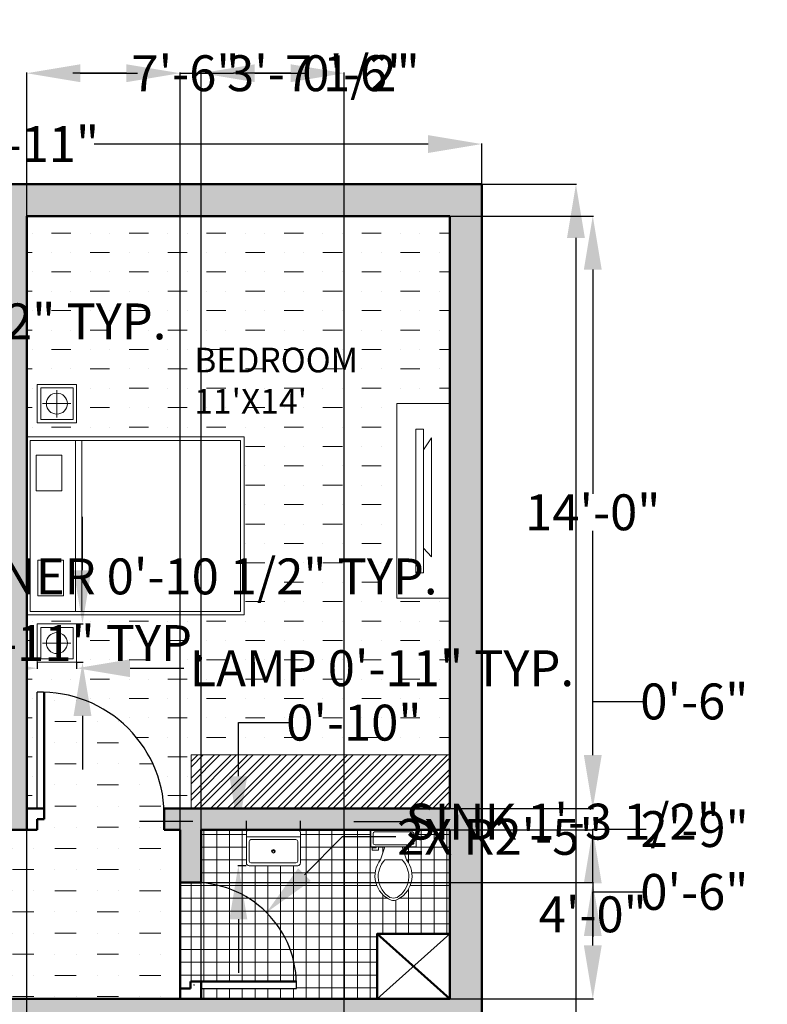
# Model space of a CAD drawing. Units: inches. Extents: x 26 to 14419, y 2 to 3479.
# Tile 5 of 9: x 13791 to 14003, y 3199 to 3479. Entities that reach past the tile are written whole.
import ezdxf

# ---------------------------------------------------------------- set-up
doc = ezdxf.new("R2010")
doc.units = ezdxf.units.IN
doc.header["$MEASUREMENT"] = 0
for name, color, linetype, lineweight in [('A-ANNO-DIMS', 2, 'Continuous', 18), ('A-AREA-IDEN', 7, 'Continuous', 18), ('A-DOOR', 4, 'Continuous', 25), ('A-FLOR-FIXT', 8, 'Continuous', 18), ('A-FLOR-PATT', 252, 'Continuous', 13), ('A-FURN', 8, 'Continuous', 18), ('A-WALL', 7, 'Continuous', 50)]:
    doc.layers.add(name, color=color, linetype=linetype, lineweight=lineweight)
doc.styles.get("Standard").update_dxf_attribs({"font": 'arial.ttf'})
doc.dimstyles.get("Standard").update_dxf_attribs({"dimtxt": 10.18, "dimasz": 15.18, "dimexe": 0.18, "dimexo": 0.0625, "dimgap": 0.09, "dimtad": 0, "dimtih": 1, "dimtoh": 1, "dimdec": 0, "dimzin": 0, "dimdsep": 46, "dimlunit": 3, "dimtxsty": 'Standard', "dimcen": 0.09, "dimadec": 0, "dimazin": 0, "dimtfac": 1, "dimtdec": 0, "dimtofl": 0, "dimtmove": 0, "dimatfit": 3, "dimfxl": 1, "dimtolj": 1, "dimtzin": 0, "dimarcsym": 0})
pattern_1 = [(0, (61.0932, 57.669), (0, 3.625), []), (90, (61.0932, 57.669), (-3.625, 2e-16), [])]

# ---------------------------------------------------------------- blocks, each defined once
blk = doc.blocks.new('*U2')
for p, q in [((9.5, -6), (9.5, -2)), ((-10, -8.5), (-8, -8.5)), ((-10, -9.5), (-10, -8.5)), ((-8, -8.5), (-8, -8)), ((-7, -8), (-7, -9.5)), ((-4, -8), (-6, -14)), ((4, -8), (6, -14)), ((-7, -9.5), (-10, -9.5)), ((4, -14), (-4, -14))]:
    blk.add_line(p, q)
blk.add_lwpolyline([(10.5, -8), (10.5, 0), (-10.5, 0), (-10.5, -8)], close=True)
for points in [[(-9.5, -2), (-9.5, -6)], [(8.5, -1), (-8.5, -1)], [(-8.5, -7), (8.5, -7)]]:
    blk.add_lwpolyline(points)
for centre, radius, start, end in [((-8.62, -1.88), 0.884, 81.8699, 188.1301), ((8.62, -1.88), 0.884, 351.8699, 98.1301), ((-8.62, -6.12), 0.884, 171.8699, 278.1301), ((8.62, -6.12), 0.884, 261.8699, 8.1301), ((3.52, -21.58), 12.17, 141.4691, 247.9714), ((4.2, -21.82), 11.33, 136.3677, 238.9468), ((-3.52, -21.58), 12.17, 292.0284, 38.5307), ((-4.2, -21.82), 11.33, 301.053, 43.6321), ((0, -27.88), 4, 245.7318, 294.2682), ((0, -29), 4, 254.8605, 285.1395)]:
    blk.add_arc(centre, radius, start, end)
blk = doc.blocks.new('Sink-single - 30 in top')
blk.add_line((-15, -3.999996), (15, -3.999996))
for points in [[(-13.5, 0), (13.5, 0)], [(-15, -18.499996), (-15, -1.5)], [(15, -1.5), (15, -18.499996)], [(-13.5, -17.499996), (-13.5, -6.499996)], [(-12.5, -5.499996), (12.5, -5.499996)], [(13.5, -6.499996), (13.5, -17.499996)], [(13.5, -19.999996), (-13.5, -19.999996)], [(12.5, -18.499996), (-12.5, -18.499996)]]:
    blk.add_lwpolyline(points)
for radius in [1, 0.5]:
    blk.add_circle((0, -11.999996), radius)
for centre, radius, start, end in [((-13.5, -1.5), 1.5, 90, 180), ((13.5, -1.5), 1.5, 0, 90), ((-12.5, -6.499996), 1, 90, 180), ((12.5, -6.499996), 1, 0, 90), ((-13.5, -18.499996), 1.5, 180, 270), ((-12.5, -17.499996), 1, 180, 270), ((12.5, -17.499996), 1, 270, 0), ((13.5, -18.499996), 1.5, 270, 0)]:
    blk.add_arc(centre, radius, start, end)
blk = doc.blocks.new('*D6')
at = {"layer": 'A-ANNO-DIMS', "color": 0, "lineweight": -2, "transparency": 16777216}
for p, q in [((13659.09, 3432.06), (13659.09, 3443.59)), ((13674.27, 3443.41), (13768.97, 3443.41)), ((13906.91, 3443.41), (13812.21, 3443.41)), ((13922.09, 3432.06), (13922.09, 3443.59))]:
    blk.add_line(p, q, dxfattribs=at)
at = {"layer": 'A-ANNO-DIMS', "color": 0, "transparency": 16777216}
for points in [[(13674.27, 3445.94), (13674.27, 3440.88), (13659.09, 3443.41)], [(13906.91, 3445.94), (13906.91, 3440.88), (13922.09, 3443.41)]]:
    blk.add_solid(points, dxfattribs=at)
at = {"layer": 'Defpoints', "color": 0, "transparency": 16777216}
for p in [(13922.09, 3443.41), (13659.09, 3432), (13922.09, 3432)]:
    blk.add_point(p, dxfattribs=at)
at = {"layer": 'A-ANNO-DIMS', "color": 0, "transparency": 16777216, "insert": (13790.59, 3443.41), "char_height": 10.18, "attachment_point": 5}
blk.add_mtext('\\A1;21\'-11"', dxfattribs=at)
blk = doc.blocks.new('*D7')
at = {"layer": 'A-ANNO-DIMS', "color": 0, "lineweight": -2, "transparency": 16777216}
for p, q in [((13922.15, 3432), (13949, 3432)), ((13948.82, 3416.82), (13948.82, 3142.28)), ((13948.82, 2857.18), (13948.82, 3131.71)), ((13922.15, 2842), (13949, 2842))]:
    blk.add_line(p, q, dxfattribs=at)
at = {"layer": 'A-ANNO-DIMS', "color": 0, "transparency": 16777216}
for points in [[(13946.29, 3416.82), (13951.35, 3416.82), (13948.82, 3432)], [(13946.29, 2857.18), (13951.35, 2857.18), (13948.82, 2842)]]:
    blk.add_solid(points, dxfattribs=at)
at = {"layer": 'Defpoints', "color": 0, "transparency": 16777216}
for p in [(13922.09, 3432), (13922.09, 2842), (13948.82, 2842)]:
    blk.add_point(p, dxfattribs=at)
at = {"layer": 'A-ANNO-DIMS', "color": 0, "transparency": 16777216, "insert": (13948.82, 3137), "char_height": 10.18, "attachment_point": 5}
blk.add_mtext('\\A1;49\'-2"', dxfattribs=at)
blk = doc.blocks.new('DOOR-900')
blk.add_line((0, 3), (0, 36))
blk.add_arc((1, 1), 35.01, 358.3634, 91.6366)
blk = doc.blocks.new('DOOR-750')
blk.add_line((3, 0), (30, 0))
blk.add_arc((1, 1), 29.02, 358.0251, 91.9749)
blk = doc.blocks.new('LAMP')
for p, q in [((5.59, 9.24), (5.59, 1.57)), ((1.47, 5.46), (9.59, 5.46))]:
    blk.add_line(p, q)
for points in [[(0, 10.91), (11.18, 10.91), (11.18, 0), (0, 0)], [(1, 9.91), (10.18, 9.91), (10.18, 1), (1, 1)]]:
    blk.add_lwpolyline(points, close=True)
blk.add_circle((5.59, 5.46), 2.98)
blk = doc.blocks.new('*D24')
at = {"layer": 'A-ANNO-DIMS', "color": 0, "lineweight": -2, "transparency": 16777216}
for p, q in [((13730.53, 3172.73), (13730.53, 3187.91)), ((13730.53, 3187.91), (13745.71, 3187.91)), ((13728.71, 3157.55), (13730.71, 3157.55)), ((13728.71, 3147.87), (13730.71, 3147.87)), ((13730.53, 3132.69), (13730.53, 3117.51))]:
    blk.add_line(p, q, dxfattribs=at)
at = {"layer": 'A-ANNO-DIMS', "color": 0, "transparency": 16777216}
for points in [[(13728, 3172.73), (13733.06, 3172.73), (13730.53, 3157.55)], [(13728, 3132.69), (13733.06, 3132.69), (13730.53, 3147.87)]]:
    blk.add_solid(points, dxfattribs=at)
at = {"layer": 'Defpoints', "color": 0, "transparency": 16777216}
for p in [(13728.65, 3157.55), (13730.53, 3157.55), (13728.65, 3147.87)]:
    blk.add_point(p, dxfattribs=at)
at = {"layer": 'A-ANNO-DIMS', "color": 0, "transparency": 16777216, "insert": (13788.69, 3187.91), "char_height": 10.18, "attachment_point": 5}
blk.add_mtext('\\A1;0\'-9 1/2" TYP.', dxfattribs=at)
blk = doc.blocks.new('*D27')
at = {"layer": 'A-ANNO-DIMS', "color": 0, "lineweight": -2, "transparency": 16777216}
for p, q in [((13755.48, 3423.45), (13755.48, 3438.63)), ((13751.01, 3408.27), (13755.66, 3408.27)), ((13751.01, 3378), (13755.66, 3378)), ((13755.48, 3362.82), (13755.48, 3347.64))]:
    blk.add_line(p, q, dxfattribs=at)
at = {"layer": 'A-ANNO-DIMS', "color": 0, "transparency": 16777216}
for points in [[(13752.95, 3423.45), (13758.01, 3423.45), (13755.48, 3408.27)], [(13752.95, 3362.82), (13758.01, 3362.82), (13755.48, 3378)]]:
    blk.add_solid(points, dxfattribs=at)
at = {"layer": 'Defpoints', "color": 0, "transparency": 16777216}
for p in [(13750.94, 3408.27), (13755.48, 3408.27), (13750.94, 3378)]:
    blk.add_point(p, dxfattribs=at)
at = {"layer": 'A-ANNO-DIMS', "color": 0, "transparency": 16777216, "insert": (13755.48, 3393.13), "char_height": 10.18, "attachment_point": 5}
blk.add_mtext('\\A1;DOOR 750 2\'-6 1/2" TYP.', dxfattribs=at)
blk = doc.blocks.new('*D35')
at = {"layer": 'A-ANNO-DIMS', "color": 0, "lineweight": -2, "transparency": 16777216}
for p, q in [((13780.88, 3294.79), (13765.7, 3294.79)), ((13796.06, 3296.4), (13796.06, 3294.61)), ((13807.24, 3296.4), (13807.24, 3294.61)), ((13822.42, 3294.79), (13837.6, 3294.79))]:
    blk.add_line(p, q, dxfattribs=at)
at = {"layer": 'A-ANNO-DIMS', "color": 0, "transparency": 16777216}
for points in [[(13780.88, 3297.32), (13780.88, 3292.26), (13796.06, 3294.79)], [(13822.42, 3297.32), (13822.42, 3292.26), (13807.24, 3294.79)]]:
    blk.add_solid(points, dxfattribs=at)
at = {"layer": 'Defpoints', "color": 0, "transparency": 16777216}
for p in [(13796.06, 3296.46), (13807.24, 3296.46), (13807.24, 3294.79)]:
    blk.add_point(p, dxfattribs=at)
at = {"layer": 'A-ANNO-DIMS', "color": 0, "transparency": 16777216, "insert": (13893.78, 3294.79), "char_height": 10.18, "attachment_point": 5}
blk.add_mtext('\\A1;LAMP 0\'-11" TYP.', dxfattribs=at)
blk = doc.blocks.new('*D36')
at = {"layer": 'A-ANNO-DIMS', "color": 0, "lineweight": -2, "transparency": 16777216}
for p, q in [((13808.91, 3322.56), (13808.91, 3337.74)), ((13807.3, 3307.38), (13809.09, 3307.38)), ((13807.3, 3296.46), (13809.09, 3296.46)), ((13808.91, 3281.28), (13808.91, 3266.1))]:
    blk.add_line(p, q, dxfattribs=at)
at = {"layer": 'A-ANNO-DIMS', "color": 0, "transparency": 16777216}
for points in [[(13806.38, 3322.56), (13811.44, 3322.56), (13808.91, 3307.38)], [(13806.38, 3281.28), (13811.44, 3281.28), (13808.91, 3296.46)]]:
    blk.add_solid(points, dxfattribs=at)
at = {"layer": 'Defpoints', "color": 0, "transparency": 16777216}
for p in [(13807.24, 3307.38), (13808.91, 3307.38), (13807.24, 3296.46)]:
    blk.add_point(p, dxfattribs=at)
at = {"layer": 'A-ANNO-DIMS', "color": 0, "transparency": 16777216, "insert": (13808.91, 3301.92), "char_height": 10.18, "attachment_point": 5}
blk.add_mtext('\\A1;0\'-11" TYP.', dxfattribs=at)
blk = doc.blocks.new('*D47')
at = {"layer": 'A-ANNO-DIMS', "color": 0, "lineweight": -2, "transparency": 16777216}
for p, q in [((13680.17, 3322.36), (13680.17, 3320.64)), ((13690.89, 3322.36), (13690.89, 3320.64)), ((13664.99, 3320.82), (13649.81, 3320.82)), ((13706.07, 3320.82), (13721.25, 3320.82))]:
    blk.add_line(p, q, dxfattribs=at)
at = {"layer": 'A-ANNO-DIMS', "color": 0, "transparency": 16777216}
for points in [[(13664.99, 3323.35), (13664.99, 3318.29), (13680.17, 3320.82)], [(13706.07, 3323.35), (13706.07, 3318.29), (13690.89, 3320.82)]]:
    blk.add_solid(points, dxfattribs=at)
at = {"layer": 'Defpoints', "color": 0, "transparency": 16777216}
for p in [(13680.17, 3322.43), (13690.89, 3322.43), (13690.89, 3320.82)]:
    blk.add_point(p, dxfattribs=at)
at = {"layer": 'A-ANNO-DIMS', "color": 0, "transparency": 16777216, "insert": (13817.29, 3320.82), "char_height": 10.18, "attachment_point": 5}
blk.add_mtext('\\A1;HOB BURNER 0\'-10 1/2" TYP.', dxfattribs=at)
blk = doc.blocks.new('*D49')
at = {"layer": 'A-ANNO-DIMS', "color": 0, "lineweight": -2, "transparency": 16777216}
for p, q in [((13840.22, 3251.29), (13825.04, 3251.29)), ((13855.4, 3249.06), (13855.4, 3251.47)), ((13870.71, 3249.06), (13870.71, 3251.47)), ((13885.89, 3251.29), (13901.07, 3251.29))]:
    blk.add_line(p, q, dxfattribs=at)
at = {"layer": 'A-ANNO-DIMS', "color": 0, "transparency": 16777216}
for points in [[(13840.22, 3253.82), (13840.22, 3248.76), (13855.4, 3251.29)], [(13885.89, 3253.82), (13885.89, 3248.76), (13870.71, 3251.29)]]:
    blk.add_solid(points, dxfattribs=at)
at = {"layer": 'Defpoints', "color": 0, "transparency": 16777216}
for p in [(13870.71, 3251.29), (13855.4, 3249), (13870.71, 3249)]:
    blk.add_point(p, dxfattribs=at)
at = {"layer": 'A-ANNO-DIMS', "color": 0, "transparency": 16777216, "insert": (13945.09, 3251.29), "char_height": 10.18, "attachment_point": 5}
blk.add_mtext('\\A1;SINK 1\'-3 1/2"', dxfattribs=at)
blk = doc.blocks.new('*D50')
at = {"layer": 'A-ANNO-DIMS', "color": 0, "lineweight": -2, "transparency": 16777216}
for p, q in [((13853.1, 3264.18), (13853.1, 3279.36)), ((13853.1, 3279.36), (13868.28, 3279.36)), ((13855.34, 3249), (13852.92, 3249)), ((13855.34, 3238.79), (13852.92, 3238.79)), ((13853.1, 3223.61), (13853.1, 3208.43))]:
    blk.add_line(p, q, dxfattribs=at)
at = {"layer": 'A-ANNO-DIMS', "color": 0, "transparency": 16777216}
for points in [[(13850.57, 3264.18), (13855.63, 3264.18), (13853.1, 3249)], [(13850.57, 3223.61), (13855.63, 3223.61), (13853.1, 3238.79)]]:
    blk.add_solid(points, dxfattribs=at)
at = {"layer": 'Defpoints', "color": 0, "transparency": 16777216}
for p in [(13853.1, 3249), (13855.4, 3249), (13855.4, 3238.79)]:
    blk.add_point(p, dxfattribs=at)
at = {"layer": 'A-ANNO-DIMS', "color": 0, "transparency": 16777216, "insert": (13885.86, 3279.36), "char_height": 10.18, "attachment_point": 5}
blk.add_mtext('\\A1;0\'-10"', dxfattribs=at)
blk = doc.blocks.new('*D68')
at = {"layer": 'A-ANNO-DIMS', "color": 0, "lineweight": -2, "transparency": 16777216}
for p, q in [((13953.59, 3216.18), (13953.59, 3231.36)), ((13953.59, 3231.36), (13968.77, 3231.36)), ((13913.15, 3201), (13953.77, 3201)), ((13913.15, 3195), (13953.77, 3195)), ((13953.59, 3179.82), (13953.59, 3164.64))]:
    blk.add_line(p, q, dxfattribs=at)
at = {"layer": 'A-ANNO-DIMS', "color": 0, "transparency": 16777216}
for points in [[(13951.06, 3216.18), (13956.12, 3216.18), (13953.59, 3201)], [(13951.06, 3179.82), (13956.12, 3179.82), (13953.59, 3195)]]:
    blk.add_solid(points, dxfattribs=at)
at = {"layer": 'Defpoints', "color": 0, "transparency": 16777216}
for p in [(13913.09, 3201), (13953.59, 3201), (13913.09, 3195)]:
    blk.add_point(p, dxfattribs=at)
at = {"layer": 'A-ANNO-DIMS', "color": 0, "transparency": 16777216, "insert": (13982.39, 3231.36), "char_height": 10.18, "attachment_point": 5}
blk.add_mtext('\\A1;0\'-6"', dxfattribs=at)
blk = doc.blocks.new('*D69')
at = {"layer": 'A-ANNO-DIMS', "color": 0, "lineweight": -2, "transparency": 16777216}
for p, q in [((13913.15, 3249), (13953.77, 3249)), ((13953.59, 3233.82), (13953.59, 3230.28)), ((13953.59, 3216.18), (13953.59, 3219.71)), ((13913.15, 3201), (13953.77, 3201))]:
    blk.add_line(p, q, dxfattribs=at)
at = {"layer": 'A-ANNO-DIMS', "color": 0, "transparency": 16777216}
for points in [[(13951.06, 3233.82), (13956.12, 3233.82), (13953.59, 3249)], [(13951.06, 3216.18), (13956.12, 3216.18), (13953.59, 3201)]]:
    blk.add_solid(points, dxfattribs=at)
at = {"layer": 'Defpoints', "color": 0, "transparency": 16777216}
for p in [(13913.09, 3249), (13953.59, 3249), (13913.09, 3201)]:
    blk.add_point(p, dxfattribs=at)
at = {"layer": 'A-ANNO-DIMS', "color": 0, "transparency": 16777216, "insert": (13953.59, 3225), "char_height": 10.18, "attachment_point": 5}
blk.add_mtext('\\A1;4\'-0"', dxfattribs=at)
blk = doc.blocks.new('*D70')
at = {"layer": 'A-ANNO-DIMS', "color": 0, "lineweight": -2, "transparency": 16777216}
for p, q in [((13953.59, 3270.18), (13953.59, 3285.36)), ((13953.59, 3285.36), (13968.77, 3285.36)), ((13913.15, 3255), (13953.77, 3255)), ((13913.15, 3249), (13953.77, 3249)), ((13953.59, 3233.82), (13953.59, 3218.64))]:
    blk.add_line(p, q, dxfattribs=at)
at = {"layer": 'A-ANNO-DIMS', "color": 0, "transparency": 16777216}
for points in [[(13951.06, 3270.18), (13956.12, 3270.18), (13953.59, 3255)], [(13951.06, 3233.82), (13956.12, 3233.82), (13953.59, 3249)]]:
    blk.add_solid(points, dxfattribs=at)
at = {"layer": 'Defpoints', "color": 0, "transparency": 16777216}
for p in [(13913.09, 3255), (13953.59, 3255), (13913.09, 3249)]:
    blk.add_point(p, dxfattribs=at)
at = {"layer": 'A-ANNO-DIMS', "color": 0, "transparency": 16777216, "insert": (13982.39, 3285.36), "char_height": 10.18, "attachment_point": 5}
blk.add_mtext('\\A1;0\'-6"', dxfattribs=at)
blk = doc.blocks.new('*D71')
at = {"layer": 'A-ANNO-DIMS', "color": 0, "lineweight": -2, "transparency": 16777216}
for p, q in [((13913.15, 3423), (13953.77, 3423)), ((13953.59, 3407.82), (13953.59, 3344.28)), ((13953.59, 3270.18), (13953.59, 3333.71)), ((13913.15, 3255), (13953.77, 3255))]:
    blk.add_line(p, q, dxfattribs=at)
at = {"layer": 'A-ANNO-DIMS', "color": 0, "transparency": 16777216}
for points in [[(13951.06, 3407.82), (13956.12, 3407.82), (13953.59, 3423)], [(13951.06, 3270.18), (13956.12, 3270.18), (13953.59, 3255)]]:
    blk.add_solid(points, dxfattribs=at)
at = {"layer": 'Defpoints', "color": 0, "transparency": 16777216}
for p in [(13913.09, 3423), (13953.59, 3423), (13913.09, 3255)]:
    blk.add_point(p, dxfattribs=at)
at = {"layer": 'A-ANNO-DIMS', "color": 0, "transparency": 16777216, "insert": (13953.59, 3339), "char_height": 10.18, "attachment_point": 5}
blk.add_mtext('\\A1;14\'-0"', dxfattribs=at)
blk = doc.blocks.new('*D78')
at = {"layer": 'A-ANNO-DIMS', "color": 0, "lineweight": -2, "transparency": 16777216}
for p, q in [((13793.09, 3201.06), (13793.09, 3463.68)), ((13808.27, 3463.5), (13821.39, 3463.5)), ((13836.57, 3201.06), (13836.57, 3463.68)), ((13836.57, 3463.5), (13851.75, 3463.5))]:
    blk.add_line(p, q, dxfattribs=at)
at = {"layer": 'A-ANNO-DIMS', "color": 0, "transparency": 16777216}
for points in [[(13808.27, 3466.03), (13808.27, 3460.97), (13793.09, 3463.5)], [(13821.39, 3466.03), (13821.39, 3460.97), (13836.57, 3463.5)]]:
    blk.add_solid(points, dxfattribs=at)
at = {"layer": 'Defpoints', "color": 0, "transparency": 16777216}
for p in [(13836.57, 3463.5), (13793.09, 3201), (13836.57, 3201)]:
    blk.add_point(p, dxfattribs=at)
at = {"layer": 'A-ANNO-DIMS', "color": 0, "transparency": 16777216, "insert": (13877.22, 3463.5), "char_height": 10.18, "attachment_point": 5}
blk.add_mtext('\\A1;3\'-7 1/2"', dxfattribs=at)
blk = doc.blocks.new('*D79')
at = {"layer": 'A-ANNO-DIMS', "color": 0, "lineweight": -2, "transparency": 16777216}
for p, q in [((13821.39, 3463.5), (13806.21, 3463.5)), ((13836.57, 3201.06), (13836.57, 3463.68)), ((13842.57, 3201.06), (13842.57, 3463.68)), ((13857.75, 3463.5), (13872.93, 3463.5))]:
    blk.add_line(p, q, dxfattribs=at)
at = {"layer": 'A-ANNO-DIMS', "color": 0, "transparency": 16777216}
for points in [[(13821.39, 3466.03), (13821.39, 3460.97), (13836.57, 3463.5)], [(13857.75, 3466.03), (13857.75, 3460.97), (13842.57, 3463.5)]]:
    blk.add_solid(points, dxfattribs=at)
at = {"layer": 'Defpoints', "color": 0, "transparency": 16777216}
for p in [(13842.57, 3463.5), (13836.57, 3201), (13842.57, 3201)]:
    blk.add_point(p, dxfattribs=at)
at = {"layer": 'A-ANNO-DIMS', "color": 0, "transparency": 16777216, "insert": (13886.55, 3463.5), "char_height": 10.18, "attachment_point": 5}
blk.add_mtext('\\A1;0\'-6"', dxfattribs=at)
blk = doc.blocks.new('*D80')
at = {"layer": 'A-ANNO-DIMS', "color": 0, "lineweight": -2, "transparency": 16777216}
for p, q in [((13953.59, 3234), (13953.59, 3249.18)), ((13953.59, 3249.18), (13968.77, 3249.18)), ((13836.63, 3234), (13953.77, 3234)), ((13953.59, 3216.18), (13953.59, 3218.82)), ((13836.63, 3201), (13953.77, 3201))]:
    blk.add_line(p, q, dxfattribs=at)
at = {"layer": 'A-ANNO-DIMS', "color": 0, "transparency": 16777216}
for points in [[(13951.06, 3218.82), (13956.12, 3218.82), (13953.59, 3234)], [(13951.06, 3216.18), (13956.12, 3216.18), (13953.59, 3201)]]:
    blk.add_solid(points, dxfattribs=at)
at = {"layer": 'Defpoints', "color": 0, "transparency": 16777216}
for p in [(13836.57, 3234), (13953.59, 3234), (13836.57, 3201)]:
    blk.add_point(p, dxfattribs=at)
at = {"layer": 'A-ANNO-DIMS', "color": 0, "transparency": 16777216, "insert": (13982.48, 3249.18), "char_height": 10.18, "attachment_point": 5}
blk.add_mtext('\\A1;2\'-9"', dxfattribs=at)
blk = doc.blocks.new('*D81')
at = {"layer": 'A-ANNO-DIMS', "color": 0, "lineweight": -2, "transparency": 16777216}
for p, q in [((13793.09, 3195.06), (13793.09, 3463.68)), ((13808.27, 3463.5), (13824.54, 3463.5)), ((13867.96, 3463.5), (13851.69, 3463.5)), ((13883.14, 3195.06), (13883.14, 3463.68))]:
    blk.add_line(p, q, dxfattribs=at)
at = {"layer": 'A-ANNO-DIMS', "color": 0, "transparency": 16777216}
for points in [[(13808.27, 3466.03), (13808.27, 3460.97), (13793.09, 3463.5)], [(13867.96, 3466.03), (13867.96, 3460.97), (13883.14, 3463.5)]]:
    blk.add_solid(points, dxfattribs=at)
at = {"layer": 'Defpoints', "color": 0, "transparency": 16777216}
for p in [(13883.14, 3463.5), (13793.09, 3195), (13883.14, 3195)]:
    blk.add_point(p, dxfattribs=at)
at = {"layer": 'A-ANNO-DIMS', "color": 0, "transparency": 16777216, "insert": (13838.12, 3463.5), "char_height": 10.18, "attachment_point": 5}
blk.add_mtext('\\A1;7\'-6"', dxfattribs=at)
blk = doc.blocks.new('*D122')
at = {"layer": 'A-ANNO-DIMS', "color": 0, "lineweight": -2, "transparency": 16777216}
for p, q in [((13882.55, 3246.98), (13871.82, 3236.25)), ((13897.73, 3246.98), (13882.55, 3246.98)), ((13840.57, 3204.91), (13840.57, 3205.09)), ((13840.48, 3205), (13840.66, 3205))]:
    blk.add_line(p, q, dxfattribs=at)
at = {"layer": 'A-ANNO-DIMS', "color": 0, "transparency": 16777216}
blk.add_solid([(13870.03, 3238.04), (13873.61, 3234.46), (13861.08, 3225.51)], dxfattribs=at)
at = {"layer": 'Defpoints', "color": 0, "transparency": 16777216}
for p in [(13861.08, 3225.51), (13840.57, 3205)]:
    blk.add_point(p, dxfattribs=at)
at = {"layer": 'A-ANNO-DIMS', "color": 0, "transparency": 16777216, "insert": (13927.25, 3246.98), "char_height": 10.18, "attachment_point": 5}
blk.add_mtext('\\A1;2X R2\'-5"', dxfattribs=at)

msp = doc.modelspace()

# ---------------------------------------------------------------- hatches: boundary and pattern name
at = {"layer": 'A-FLOR-PATT'}
h = msp.add_hatch(color=256, dxfattribs=at)
h.dxf.hatch_style = 1
h.paths.add_polyline_path([(13922.09, 3432), (13659.09, 3432), (13659.09, 2842), (13668.09, 2842), (13668.09, 2851), (13668.09, 2899), (13668.09, 2908), (13668.09, 3076), (13706.09, 3076), (13706.09, 3085), (13668.09, 3085), (13668.09, 3249), (13712.76, 3249), (13712.76, 3255), (13668.09, 3255), (13668.09, 3375), (13720.94, 3375), (13720.94, 3378, -0.017236), (13720.94, 3380), (13720.94, 3381), (13668.09, 3381), (13668.09, 3423), (13784.09, 3423), (13784.09, 3381), (13753.94, 3381), (13753.94, 3375), (13784.09, 3375), (13784.09, 3255), (13758.77, 3255), (13758.77, 3249), (13784.09, 3249), (13793.09, 3249), (13793.09, 3255), (13793.09, 3423), (13913.09, 3423), (13913.09, 3255), (13832.09, 3255), (13832.09, 3254, -0.014283), (13832.09, 3252), (13832.09, 3249), (13836.57, 3249), (13836.57, 3234), (13839.57, 3234, -0.017236), (13841.57, 3234), (13842.57, 3234), (13842.57, 3249), (13913.09, 3249), (13913.09, 3201), (13892.46, 3201), (13793.09, 3201), (13784.09, 3201), (13784.09, 3195), (13793.09, 3195), (13913.09, 3195), (13913.09, 3127), (13922.09, 3127)])
h.paths.add_polyline_path([(13922.09, 3013.5), (13913.09, 3013.5), (13913.09, 2908), (13892.09, 2908), (13892.09, 2899), (13913.09, 2899), (13913.09, 2851), (13793.09, 2851), (13784.09, 2851), (13784.09, 2842), (13922.09, 2842)], flags=17)
h.paths.add_polyline_path([(13793.09, 3085), (13784.09, 3085), (13784.09, 3076), (13784.09, 3071.08), (13784.09, 3066.17), (13784.09, 2908), (13784.09, 2899.07), (13793.09, 2899), (13802.09, 2899), (13814.09, 2899), (13814.09, 2908), (13793.09, 2908)], flags=17)
h.paths.add_polyline_path([(14342.64, 3401.72), (14242.78, 3401.72), (14242.78, 3392.72), (14257.64, 3392.72), (14257.64, 3351.75), (14257.64, 3345.75), (14257.64, 3330.73), (14263.64, 3330.73), (14263.64, 3392.72), (14333.64, 3392.72), (14333.64, 3284.72), (14302.92, 3284.72), (14302.92, 3281.72, -0.022645), (14302.92, 3279.12), (14302.92, 3278.72), (14333.64, 3278.72), (14333.64, 3170.72), (14316.1, 3170.72), (14263.64, 3170.72), (14263.64, 3278.72), (14269.92, 3278.72), (14269.92, 3284.72), (14263.64, 3284.72), (14257.64, 3284.72), (14257.64, 3225.75), (14257.64, 3219.75), (14257.64, 3164.72), (14333.64, 3164.72), (14333.64, 3110.37), (14210.01, 3110.37), (14210.01, 3104.37), (14257.64, 3104.37), (14257.64, 3024), (14263.64, 3024), (14263.64, 3039.72), (14263.64, 3104.37), (14333.64, 3104.37), (14333.64, 3045.72), (14333.64, 3039.72), (14333.64, 2967.72), (14296.64, 2967.72), (14296.64, 2964.72, -0.017236), (14296.64, 2962.72), (14296.64, 2961.72), (14333.64, 2961.72), (14333.64, 2882.72), (14312.64, 2882.72), (14312.64, 2873.72), (14333.64, 2873.72), (14333.64, 2820.72), (14333.64, 2811.72), (14342.64, 2811.72)])
h.paths.add_polyline_path([(14088.64, 3219.75), (14218.64, 3219.75), (14218.64, 3222.75, -0.014283), (14218.64, 3224.75), (14218.64, 3225.75), (14088.64, 3225.75), (14088.64, 3345.75), (14088.64, 3351.75), (14088.64, 3392.72), (14193.93, 3392.72), (14193.93, 3351.75), (14140.64, 3351.75), (14140.64, 3345.75), (14170.7, 3345.75), (14218.64, 3345.75), (14218.64, 3348.75, -0.014283), (14218.64, 3350.75), (14218.64, 3351.75), (14199.93, 3351.75), (14199.93, 3392.72), (14214.78, 3392.72), (14214.78, 3401.72), (14079.64, 3401.72), (14079.64, 2811.72), (14088.64, 2811.72), (14088.64, 2820.72), (14088.64, 2873.72), (14116.21, 2873.72), (14116.21, 2876.57), (14116.21, 2882.72), (14088.64, 2882.72), (14088.64, 3039.72), (14216.01, 3039.72), (14216.01, 3065.37), (14215.01, 3065.37, -0.014283), (14213.01, 3065.37), (14210.01, 3065.37), (14210.01, 3045.72), (14154.64, 3045.72), (14148.64, 3045.72), (14088.64, 3045.72)])
h.paths.add_polyline_path([(14284.64, 2882.72), (14263.64, 2882.72), (14263.64, 2961.72), (14263.64, 2967.72), (14257.64, 2967.72), (14257.64, 2956.69), (14257.64, 2916.18), (14257.64, 2882.72), (14249.61, 2882.72), (14249.61, 2873.72), (14284.64, 2873.72)], flags=17)
h.paths.add_polyline_path([(14202.78, 2882.72), (14189.55, 2882.72), (14189.55, 2879.95), (14189.55, 2873.72), (14202.78, 2873.72)], flags=17)
h = msp.add_hatch(dxfattribs=at)
h.set_pattern_fill('MUDST', color=256, scale=22)
h.set_pattern_definition([(0, (61.093, 57.669), (11, 5.5), [5.5, -5.5, 0, -5.5, 0, -5.5])])
h.paths.add_polyline_path([(13913.09, 3423), (13793.09, 3423), (13793.09, 3360.36), (13854.72, 3360.36), (13854.72, 3309.9), (13793.09, 3309.9), (13793.09, 3255), (13796.09, 3255), (13796.09, 3288, -0.405865), (13832.05, 3255), (13839.69, 3255), (13839.69, 3270.22), (13913.09, 3270.22), (13913.09, 3314.65), (13898.01, 3314.65), (13898.01, 3369.81), (13913.09, 3369.81)])
h.paths.add_polyline_path([(13807.24, 3364.35), (13796.06, 3364.35), (13796.06, 3375.26), (13807.24, 3375.26)], flags=16)
h.paths.add_polyline_path([(13806.24, 3365.35), (13797.06, 3365.35), (13797.06, 3374.26), (13806.24, 3374.26)], flags=0)
h.paths.add_polyline_path([(13804.63, 3369.81, -1), (13798.67, 3369.81, -1)], flags=0)
h.paths.add_polyline_path([(13807.24, 3307.38), (13807.24, 3296.46), (13796.06, 3296.46), (13796.06, 3307.38)], flags=16)
h.paths.add_polyline_path([(13806.24, 3306.38), (13806.24, 3297.46), (13797.06, 3297.46), (13797.06, 3306.38)], flags=0)
h.paths.add_polyline_path([(13804.63, 3301.92, -1), (13798.67, 3301.92, -1)], flags=0)
h = msp.add_hatch(dxfattribs=at)
h.set_pattern_fill('MUDST', color=256, scale=24)
h.set_pattern_definition([(0, (61.093, 57.669), (12, 6), [6, -6, 0, -6, 0, -6])])
h.paths.add_polyline_path([(13756.28, 3375), (13750.94, 3375), (13720.94, 3375), (13706.54, 3375), (13706.54, 3255), (13712.76, 3255), (13712.76, 3249), (13668.09, 3249), (13668.09, 3085), (13709.09, 3085), (13709.09, 3116.5, -0.393405), (13744.93, 3085), (13745.25, 3085, -0.393405), (13781.09, 3116.5), (13781.09, 3085), (13784.09, 3085), (13784.09, 3127), (13784.09, 3195), (13784.09, 3201), (13793.09, 3201), (13836.57, 3201), (13836.57, 3204), (13836.57, 3234), (13836.57, 3249), (13832.09, 3249), (13832.09, 3254, 0.397579), (13798.09, 3288), (13798.09, 3252), (13796.09, 3252), (13796.09, 3249), (13793.09, 3249), (13784.09, 3249), (13758.77, 3249), (13758.77, 3255), (13784.09, 3255), (13784.09, 3303.43), (13756.28, 3303.43)])
h.paths.add_polyline_path([(13757.29, 3298.63), (13757.76, 3298.12), (13779.63, 3298.12), (13779.63, 3268.87), (13757.77, 3268.87), (13756.19, 3268.87), (13756.19, 3285.02), (13757.77, 3285.02), (13757.77, 3298.11), (13749.96, 3290.89), (13749.48, 3291.4)], flags=16)
h.paths.add_polyline_path([(13758.77, 3297.12), (13778.63, 3297.12), (13778.63, 3269.87), (13758.77, 3269.87)], flags=0)
h.paths.add_polyline_path([(13716.08, 3198.11), (13716.08, 3190.37), (13728.65, 3190.37), (13728.65, 3180.68), (13716.08, 3180.68), (13716.08, 3174.63), (13728.65, 3174.63), (13728.65, 3164.95), (13716.08, 3164.95), (13716.08, 3157.55), (13728.65, 3157.55), (13728.65, 3147.87), (13716.08, 3147.87), (13716.08, 3142.39), (13687.89, 3142.39), (13687.89, 3145.78), (13675.33, 3145.78), (13675.33, 3155.46), (13687.89, 3155.46), (13687.89, 3163.27), (13675.33, 3163.27), (13675.33, 3172.95), (13687.89, 3172.95), (13687.89, 3179.58), (13675.33, 3179.58), (13675.33, 3189.26), (13687.89, 3189.26), (13687.89, 3198.11)], flags=16)
h.paths.add_polyline_path([(13715.08, 3197.11), (13715.08, 3143.39), (13688.89, 3143.39), (13688.89, 3197.11)], flags=0)
h = msp.add_hatch(dxfattribs=at)
h.set_pattern_fill('ANSI32', color=256, scale=8.9)
h.set_pattern_definition([(45, (61.0932, 57.669), (-2.3599689, 2.3599689), []), (45, (62.6665, 57.669), (-2.3599689, 2.3599689), [])])
h.paths.add_polyline_path([(13913.09, 3270.22), (13839.69, 3270.22), (13839.69, 3255), (13913.09, 3255)])
h = msp.add_hatch(dxfattribs=at)
h.set_pattern_fill('NET', color=256, scale=29)
h.set_pattern_definition(pattern_1)
h.paths.add_polyline_path([(13913.09, 3249), (13903.47, 3249), (13903.47, 3244.13), (13899.52, 3244.13), (13900.74, 3240.48, -0.501323), (13897.72, 3229.01, -0.132891), (13896.45, 3229.01, -0.501317), (13893.44, 3240.48), (13894.65, 3244.13), (13892.83, 3244.13), (13892.83, 3243.22), (13891, 3243.22), (13891, 3243.83), (13892.22, 3243.83), (13892.22, 3244.13), (13890.7, 3244.13), (13890.7, 3249), (13869.94, 3249, -0.414214), (13870.71, 3248.23), (13870.71, 3239.56, -0.414214), (13869.94, 3238.79), (13856.17, 3238.79, -0.414214), (13855.4, 3239.56), (13855.4, 3248.23, -0.414214), (13856.17, 3249), (13842.57, 3249), (13842.57, 3233.94, -0.404142), (13869.57, 3204), (13842.57, 3204), (13842.57, 3201), (13892.46, 3201), (13892.46, 3219.45), (13913.09, 3219.45)])
h = msp.add_hatch(dxfattribs=at)
h.set_pattern_fill('NET', color=256, scale=29)
h.set_pattern_definition(pattern_1)
h.paths.add_polyline_path([(13869.57, 3206), (13839.57, 3206), (13839.57, 3204), (13836.57, 3204), (13836.57, 3234), (13839.57, 3234, -0.414214)])

# ---------------------------------------------------------------- linework, layer by layer
at = {"layer": 'A-FLOR-FIXT'}
msp.add_line((13892.46, 3201), (13913.09, 3219.45), dxfattribs=at)
at = {"layer": 'A-FURN'}
for p, q in [((13806.91, 3310.9), (13806.91, 3359.36)), ((13808.7, 3310.9), (13808.7, 3359.36)), ((13808.7, 3359.36), (13815.93, 3359.36)), ((13905.62, 3356.69), (13907.9, 3360.07)), ((13907.9, 3360.07), (13907.9, 3326.35)), ((13907.9, 3326.35), (13905.62, 3328.82)), ((13839.69, 3255), (13839.69, 3270.22)), ((13839.69, 3270.22), (13913.09, 3270.22))]:
    msp.add_line(p, q, dxfattribs=at)
for points in [[(13913.09, 3369.81), (13898.01, 3369.81), (13898.01, 3314.65), (13913.09, 3314.65)], [(13905.62, 3362.58), (13903.39, 3362.58), (13903.39, 3321.81), (13905.62, 3321.81)], [(13793.09, 3360.36), (13854.72, 3360.36), (13854.72, 3309.9), (13793.09, 3309.9)], [(13794.09, 3359.36), (13853.72, 3359.36), (13853.72, 3310.9), (13794.09, 3310.9)], [(13795.77, 3355.23), (13803.03, 3355.23), (13803.03, 3345.12), (13795.77, 3345.12)], [(13796.28, 3325.41), (13803.54, 3325.41), (13803.54, 3315.3), (13796.28, 3315.3)]]:
    msp.add_lwpolyline(points, close=True, dxfattribs=at)
at = {"layer": 'A-WALL'}
for p, q in [((13659.09, 3432), (13922.09, 3432)), ((13922.09, 3432), (13922.09, 2842)), ((13793.09, 3423), (13913.09, 3423)), ((13793.09, 3255), (13793.09, 3423)), ((13913.09, 3423), (13913.09, 3255)), ((13798.09, 3252), (13798.09, 3288)), ((13793.09, 3255), (13798.09, 3255)), ((13793.09, 3255), (13793.09, 3249)), ((13832.05, 3255), (13913.09, 3255)), ((13832.09, 3255), (13832.09, 3249)), ((13796.09, 3252), (13796.09, 3249)), ((13798.09, 3252), (13796.09, 3252)), ((13784.09, 3249), (13793.09, 3249)), ((13793.09, 3249), (13796.09, 3249)), ((13832.09, 3249), (13836.57, 3249)), ((13836.57, 3249), (13836.57, 3234)), ((13842.57, 3249), (13842.57, 3233.94)), ((13842.57, 3249), (13913.09, 3249)), ((13913.09, 3249), (13913.09, 3201)), ((13836.57, 3234), (13842.57, 3234)), ((13836.57, 3234), (13836.57, 3204)), ((13892.46, 3219.45), (13913.09, 3201)), ((13839.57, 3206), (13869.57, 3206)), ((13839.57, 3206), (13839.57, 3204)), ((13842.57, 3206), (13842.57, 3201)), ((13836.57, 3204), (13839.57, 3204)), ((13836.57, 3204), (13836.57, 3201)), ((13793.09, 3201), (13784.09, 3201)), ((13793.09, 3201), (13913.09, 3201))]:
    msp.add_line(p, q, dxfattribs=at)
msp.add_lwpolyline([(13913.09, 3201), (13892.46, 3201), (13892.46, 3219.45), (13913.09, 3219.45)], close=True, dxfattribs=at)

# ---------------------------------------------------------------- block references
at = {"layer": 'A-DOOR'}
for name, p in [('DOOR-900', (13796.09, 3252)), ('DOOR-750', (13839.57, 3204))]:
    msp.add_blockref(name, p, dxfattribs=at)
at = {"layer": 'A-FLOR-FIXT'}
for name, p, xscale, yscale, zscale in [('Sink-single - 30 in top', (13863.05, 3249), 0.5101879175420303, 0.5101879175420303, 0.5101879175420303), ('*U2', (13897.09, 3249), 0.6083342517074687, 0.6083342517074687, 0.6083342517074687)]:
    msp.add_blockref(name, p, dxfattribs=dict(at, xscale=xscale, yscale=yscale, zscale=zscale))
at = {"layer": 'A-FURN'}
for p in [(13796.06, 3364.35), (13796.06, 3296.46)]:
    msp.add_blockref('LAMP', p, dxfattribs=at)

# ---------------------------------------------------------------- texts
at = {"layer": 'A-AREA-IDEN', "insert": (13840.59, 3385.67), "char_height": 7, "attachment_point": 1}
msp.add_mtext_dynamic_manual_height_columns("BEDROOM\\P11'X14'", width=51, gutter_width=1, heights=[0], dxfattribs=at)

# ---------------------------------------------------------------- dimensions: what is measured, and where the dimension line sits
at = {"layer": 'A-ANNO-DIMS'}
for base, p1, p2, override, picture, middle in [((13836.57, 3463.5), (13793.09, 3201), (13836.57, 3201), {"dimdec": 1, "dimlfac": 1, "dimrnd": 0, "dimzin": 1, "dimdsep": 46, "dimlunit": 4, "dimfrac": 2}, '*D78', (13877.22, 3463.5)), ((13883.1394, 3463.496), (13793.0912, 3194.996), (13883.1394, 3194.996), {"dimdec": 1, "dimlfac": 1, "dimrnd": 0, "dimzin": 1, "dimdsep": 46, "dimlunit": 4, "dimfrac": 2}, '*D81', (13838.1153, 3463.496)), ((13842.57, 3463.5), (13836.57, 3201), (13842.57, 3201), {"dimdec": 1, "dimlfac": 1, "dimrnd": 0, "dimzin": 1, "dimdsep": 46, "dimlunit": 4, "dimfrac": 2}, '*D79', (13886.55, 3463.5)), ((13922.09, 3443.41), (13659.09, 3432), (13922.09, 3432), {"dimclrd": 0, "dimclre": 0, "dimclrt": 0}, '*D6', (13790.59, 3443.41))]:
    dim = msp.add_linear_dim(base=base, p1=p1, p2=p2, dimstyle='Standard', override=override, dxfattribs=at)
    dim.commit()
    dim.dimension.update_dxf_attribs({"geometry": picture, "text_midpoint": middle})
for base, p1, p2, text, picture, middle in [((13755.48, 3408.27), (13750.94, 3378), (13750.94, 3408.27), 'DOOR 750 <> TYP.', '*D27', (13755.48, 3393.13)), ((13808.91, 3307.38), (13807.24, 3296.46), (13807.24, 3307.38), '<> TYP.', '*D36', (13808.91, 3301.92)), ((13730.53, 3157.55), (13728.65, 3147.87), (13728.65, 3157.55), '<> TYP.', '*D24', (13788.69, 3187.91))]:
    dim = msp.add_linear_dim(base=base, p1=p1, p2=p2, angle=90, text=text, dimstyle='Standard', override={"dimdec": 1, "dimrnd": 0, "dimzin": 1, "dimlunit": 4, "dimfrac": 2}, dxfattribs=at)
    dim.commit()
    dim.dimension.update_dxf_attribs({"geometry": picture, "text_midpoint": middle})
for base, p1, p2, override, picture, middle in [((13948.82, 2842), (13922.09, 3432), (13922.09, 2842), {"dimclrd": 0, "dimclre": 0, "dimclrt": 0}, '*D7', (13948.82, 3137)), ((13953.59, 3423), (13913.09, 3255), (13913.09, 3423), {"dimdec": 1, "dimlfac": 1, "dimrnd": 0, "dimzin": 1, "dimdsep": 46, "dimlunit": 4, "dimfrac": 2}, '*D71', (13953.59, 3339)), ((13953.59, 3255), (13913.09, 3249), (13913.09, 3255), {"dimdec": 1, "dimlfac": 1, "dimrnd": 0, "dimzin": 1, "dimdsep": 46, "dimlunit": 4, "dimfrac": 2}, '*D70', (13982.39, 3285.36)), ((13853.1, 3249), (13855.4, 3238.79), (13855.4, 3249), {"dimdec": 1, "dimrnd": 0, "dimzin": 1, "dimlunit": 4, "dimfrac": 2}, '*D50', (13885.86, 3279.36)), ((13953.59, 3234), (13836.57, 3201), (13836.57, 3234), {"dimdec": 1, "dimlfac": 1, "dimrnd": 0, "dimzin": 1, "dimdsep": 46, "dimlunit": 4, "dimfrac": 2}, '*D80', (13982.48, 3249.18)), ((13953.59, 3249), (13913.09, 3201), (13913.09, 3249), {"dimdec": 1, "dimlfac": 1, "dimrnd": 0, "dimzin": 1, "dimdsep": 46, "dimlunit": 4, "dimfrac": 2}, '*D69', (13953.59, 3225)), ((13953.59, 3201), (13913.09, 3195), (13913.09, 3201), {"dimdec": 1, "dimlfac": 1, "dimrnd": 0, "dimzin": 1, "dimdsep": 46, "dimlunit": 4, "dimfrac": 2}, '*D68', (13982.39, 3231.36))]:
    dim = msp.add_linear_dim(base=base, p1=p1, p2=p2, angle=90, dimstyle='Standard', override=override, dxfattribs=at)
    dim.commit()
    dim.dimension.update_dxf_attribs({"geometry": picture, "text_midpoint": middle})
for base, p1, p2, text, picture, middle in [((13690.89, 3320.82), (13680.17, 3322.43), (13690.89, 3322.43), 'HOB BURNER <> TYP.', '*D47', (13817.29, 3320.82)), ((13807.24, 3294.79), (13796.06, 3296.46), (13807.24, 3296.46), 'LAMP <> TYP.', '*D35', (13893.78, 3294.79)), ((13870.71, 3251.29), (13855.4, 3249), (13870.71, 3249), 'SINK <>', '*D49', (13945.09, 3251.29))]:
    dim = msp.add_linear_dim(base=base, p1=p1, p2=p2, text=text, dimstyle='Standard', override={"dimdec": 1, "dimrnd": 0, "dimzin": 1, "dimlunit": 4, "dimfrac": 2}, dxfattribs=at)
    dim.commit()
    dim.dimension.update_dxf_attribs({"geometry": picture, "text_midpoint": middle})
dim = msp.add_radius_dim(center=(13840.57, 3205), mpoint=(13861.08, 3225.51), text='2X <>', dimstyle='Standard', override={"dimdec": 1, "dimlfac": 1, "dimrnd": 0, "dimzin": 1, "dimdsep": 46, "dimlunit": 4, "dimfrac": 2}, dxfattribs=at)
dim.commit()
dim.dimension.update_dxf_attribs({"geometry": '*D122', "text_midpoint": (13927.25, 3246.98)})

doc.saveas('drawing.dxf')
